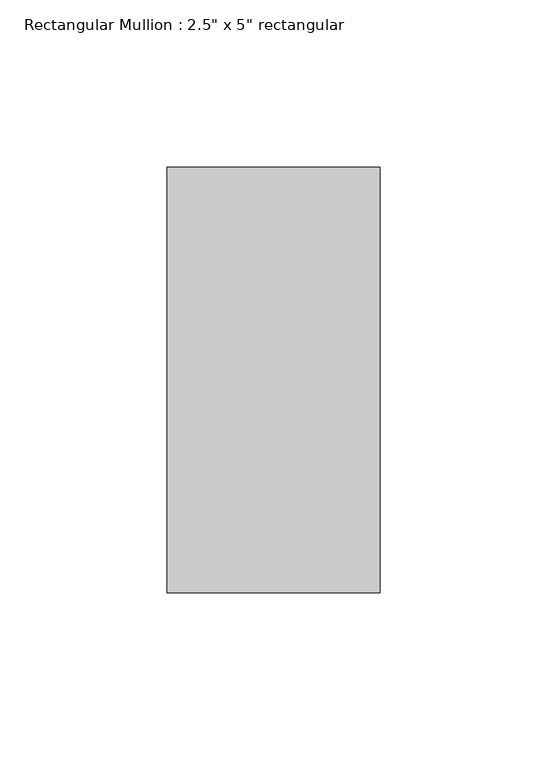
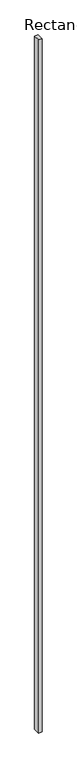
"""IFC4 building model written with IfcOpenShell, lengths in millimetres: member geometry."""

from ifc_helpers import new_model, si_unit, frame, origin, place, context, project, spatial, polyline, outline, extrude, source, transform, mapped, element, save


def member_a7b860c5(model_context):
    return source(origin(), model_context, "Body", "SweptSolid", [
        extrude(outline(polyline([(0.0, 63.5), (0.0, -63.5), (-63.5, -63.5), (-63.5, 63.5), (0.0, 63.5)])), frame((0.0, 0.0, -13669.82075), z_axis=(0.0, 0.0, 1.0), x_axis=(1.0, 0.0, 0.0)), (0.0, 0.0, 1.0), 13669.82075),
    ])


if __name__ == "__main__":
    model = new_model("IFC4")
    model_context = context("Model", 3, world=origin())
    ifc_project = project(units=[si_unit("LENGTHUNIT", "METRE", prefix="MILLI")], contexts=[model_context])
    site = spatial("IfcSite", under=ifc_project)
    building = spatial("IfcBuilding", under=site)
    placement = place(None, origin())
    member_shape = member_a7b860c5(model_context)
    element("IfcMember", 1, ObjectType="Rectangular Mullion : 2.5\" x 5\" rectangular", at=placement, inside=building, context=model_context, shape_type="MappedRepresentation", body=[
        mapped(member_shape, transform((0.0, 0.0, 0.0), x_axis=(1.0, 0.0, 0.0), y_axis=(0.0, 1.0, 0.0), z_axis=(0.0, 0.0, 1.0))),
    ])
    save(model, "model.ifc")

# Revit data of these elements
# Type "Rectangular Mullion : 2.5\" x 5\" rectangular"
#   built-in parameter 1007304 = 0.416667 (stored number, unit not read)
#   built-in parameter 1007301 = 0.104167 (stored number, unit not read)
#   built-in parameter 1007300 = 0.104167 (stored number, unit not read)
# Element 1 (IfcMember, "Rectangular Mullion : 2.5\" x 5\" rectangular")
#   Materials on its faces: "Aluminum"
# Materials
#   "Aluminum": class "Metal", colour RGB 247 247 247, transparency 0, Description = "Aluminum 6061", Cost = 0
